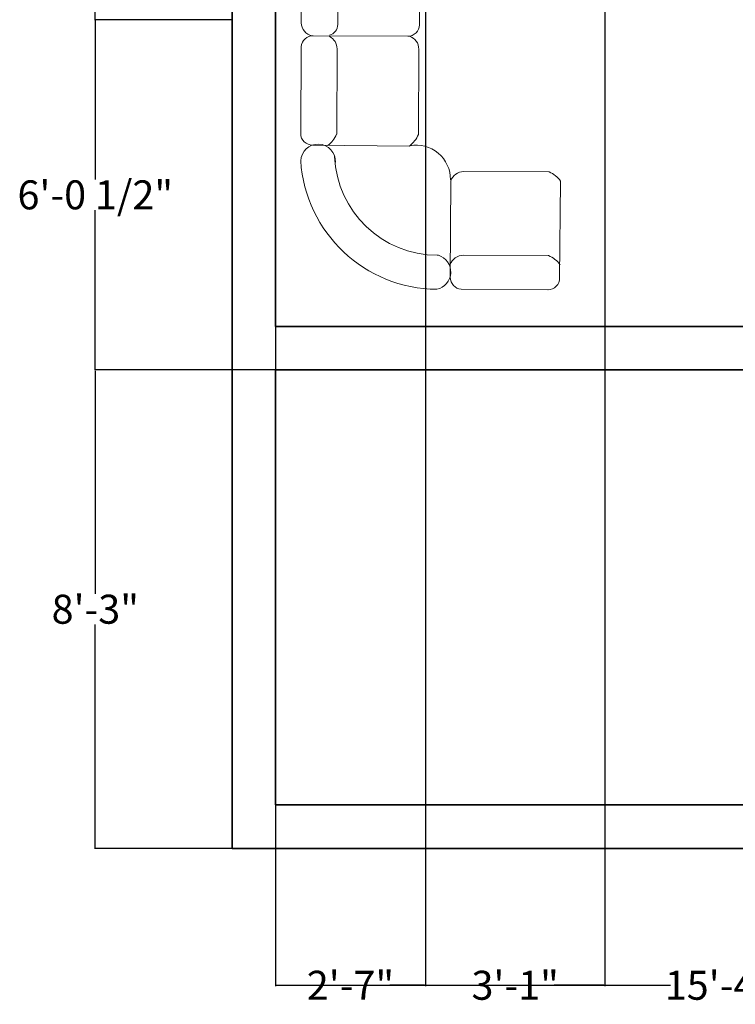
# Model space of a CAD drawing. Units: inches. Extents: x -26 to 575, y -18 to 513.
# Tile 1 of 28: x -26 to 122, y -13 to 191. Entities that reach past the tile are written whole.
import ezdxf

# ---------------------------------------------------------------- set-up
doc = ezdxf.new("R2010")
doc.units = ezdxf.units.IN
doc.header["$MEASUREMENT"] = 0
for name, color, linetype, lineweight in [('A-ANNO-DIMS', 2, 'Continuous', 18), ('A-WALL', 7, 'Continuous', 35), ('Furniture', 8, 'Continuous', 15)]:
    doc.layers.add(name, color=color, linetype=linetype, lineweight=lineweight)
doc.styles.get("Standard").update_dxf_attribs({"font": 'arial.ttf', "height": 6})
doc.dimstyles.get("Standard").update_dxf_attribs({"dimtxt": 6, "dimasz": 0.18, "dimexe": 0.18, "dimexo": 0.0625, "dimgap": 0.09, "dimtad": 0, "dimtih": 1, "dimtoh": 1, "dimzin": 0, "dimdsep": 46, "dimlunit": 3, "dimtxsty": 'Standard', "dimcen": 0.09, "dimadec": 0, "dimazin": 0, "dimtfac": 1, "dimtofl": 0, "dimtmove": 0, "dimatfit": 3, "dimfxl": 1, "dimtolj": 1, "dimtzin": 0, "dimarcsym": 0})

# ---------------------------------------------------------------- blocks, each defined once
blk = doc.blocks.new('SOFA-L-SECTIONAL')
for p, q in [((22.74, 97.99, -13.5), (2.82, 98.09, -13.5)), ((0.33, 95.83, -13.5), (0.23, 77.86, -13.5)), ((7.68, 77.72, -13.5), (7.77, 95.38, -13.5)), ((24.59, 77.63, -13.5), (24.69, 95.29, -13.5)), ((2.7, 75.47, -13.5), (22.72, 75.27, -13.5)), ((0.21, 72.7, -13.5), (0.12, 55.25, -13.5)), ((7.74, 68.12, -13.5), (7.76, 72.56, -13.5)), ((24.65, 68.03, -13.5), (24.67, 72.47, -13.5)), ((7.67, 54.9, -13.5), (7.74, 68.12, -13.5)), ((24.58, 54.81, -13.5), (24.65, 68.03, -13.5)), ((2.38, 52.55, -13.5), (22.19, 52.45, -13.5)), ((22.5, 52.45, -13.5), (2.58, 52.55, -13.5)), ((0.09, 50.29, -13.5), (0, 32.32, -13.5)), ((7.45, 32.18, -13.5), (7.54, 49.84, -13.5)), ((24.36, 32.09, -13.5), (24.45, 49.75, -13.5)), ((2.47, 29.93, -13.5), (22.49, 29.73, -13.5)), ((51.42, 24.36, -13.5), (33.76, 24.45, -13.5)), ((31.06, 22.5, -13.5), (30.96, 2.58, -13.5)), ((53.78, 22.49, -13.5), (53.58, 2.47, -13.5)), ((28.5, 7.13, -13.5), (28.26, 7.13, -13.5)), ((51.33, 7.05, -13.5), (33.67, 7.14, -13.5)), ((30.97, 5.19, -13.5), (30.97, 5.12, -13.5)), ((33.22, 0.09, -13.5), (51.19, 0, -13.5))]:
    blk.add_line(p, q)
for centre, radius, start, end in [((2.8, 95.6, -13.5), 2.49, 89.7045, 174.7543), ((4.96, 95.39, -13.5), 2.82, 359.7045, 63.7788), ((21.87, 95.31, -13.5), 2.82, 359.7045, 71.9933), ((2.61, 77.85, -13.5), 2.38, 179.7045, 272.1133), ((2.36, 80.01, -13.5), 5.79, 306.5883, 336.7547), ((19.27, 79.92, -13.5), 5.79, 306.5883, 336.7547), ((3.67, 72.1, -13.5), 3.51, 105.9725, 170.1982), ((4.8, 72.57, -13.5), 2.96, 359.7045, 69.9456), ((21.71, 72.48, -13.5), 2.96, 359.7045, 69.9456), ((2.84, 55.23, -13.5), 2.72, 179.7045, 260.1487), ((5.3, 54.91, -13.5), 2.37, 286.4623, 359.7335), ((22.21, 54.82, -13.5), 2.37, 269.7045, 359.7335), ((2.57, 50.06, -13.5), 2.49, 89.7045, 174.7543), ((4.72, 49.86, -13.5), 2.82, 359.7045, 63.7788), ((21.63, 49.77, -13.5), 2.82, 359.7045, 71.9933), ((2.38, 32.31, -13.5), 2.38, 179.7045, 272.1133), ((2.12, 34.47, -13.5), 5.79, 306.5883, 336.7547), ((19.04, 34.38, -13.5), 5.79, 306.5883, 336.7547), ((3.6, 26.52, -13.5), 3.6, 357.7166, 177.7166), ((23.89, 22.8, -13.5), 7.12, 359.7045, 100.3051), ((28.37, 28.51, -13.5), 28.42, 183.6915, 269.6528), ((28.37, 28.51, -13.5), 21.38, 182.6205, 269.7045), ((33.74, 21.63, -13.5), 2.82, 89.7045, 161.9933), ((49.13, 19.04, -13.5), 5.79, 36.5883, 66.7547), ((27.43, 3.65, -13.5), 3.64, 282.1306, 72.938), ((33.65, 4.32, -13.5), 2.82, 89.7045, 161.9933), ((49.04, 1.73, -13.5), 5.79, 36.5883, 66.7547), ((33.45, 2.57, -13.5), 2.49, 179.7045, 264.7543), ((51.2, 2.38, -13.5), 2.38, 269.7045, 2.1133)]:
    blk.add_arc(centre, radius, start, end)
blk = doc.blocks.new('*D28')
at = {"layer": 'A-ANNO-DIMS', "color": 0, "lineweight": -2, "transparency": 16777216}
for p, q in [((58.22, 466.45), (58.22, -8.97)), ((95.35, 466.45), (95.35, -8.97)), ((58.4, -8.79), (68.72, -8.79)), ((95.17, -8.79), (84.85, -8.79))]:
    blk.add_line(p, q, dxfattribs=at)
at = {"layer": 'A-ANNO-DIMS', "color": 0, "transparency": 16777216}
for points in [[(58.4, -8.76), (58.4, -8.82), (58.22, -8.79)], [(95.17, -8.76), (95.17, -8.82), (95.35, -8.79)]]:
    blk.add_solid(points, dxfattribs=at)
at = {"layer": 'Defpoints', "color": 0, "transparency": 16777216}
for p in [(58.22, 466.51), (95.35, 466.51), (95.35, -8.79)]:
    blk.add_point(p, dxfattribs=at)
at = {"layer": 'A-ANNO-DIMS', "color": 0, "transparency": 16777216, "insert": (76.79, -8.79), "char_height": 6, "attachment_point": 5}
blk.add_mtext('\\A1;3\'-1"', dxfattribs=at)
blk = doc.blocks.new('*D33')
at = {"layer": 'A-ANNO-DIMS', "color": 0, "lineweight": -2, "transparency": 16777216}
for p, q in [((27.11, 118.51), (-10.3, 118.51)), ((-10.12, 118.33), (-10.12, 72.16)), ((-10.12, 19.69), (-10.12, 65.85)), ((18.11, 19.51), (-10.3, 19.51))]:
    blk.add_line(p, q, dxfattribs=at)
at = {"layer": 'A-ANNO-DIMS', "color": 0, "transparency": 16777216}
for points in [[(-10.15, 118.33), (-10.09, 118.33), (-10.12, 118.51)], [(-10.15, 19.69), (-10.09, 19.69), (-10.12, 19.51)]]:
    blk.add_solid(points, dxfattribs=at)
at = {"layer": 'Defpoints', "color": 0, "transparency": 16777216}
for p in [(-10.12, 118.51), (27.18, 118.51), (18.18, 19.51)]:
    blk.add_point(p, dxfattribs=at)
at = {"layer": 'A-ANNO-DIMS', "color": 0, "transparency": 16777216, "insert": (-10.12, 69.01), "char_height": 6, "attachment_point": 5}
blk.add_mtext('\\A1;8\'-3"', dxfattribs=at)
blk = doc.blocks.new('*D36')
at = {"layer": 'A-ANNO-DIMS', "color": 0, "lineweight": -2, "transparency": 16777216}
for p, q in [((18.11, 267.49), (-10.3, 267.49)), ((-10.12, 267.31), (-10.12, 232.43)), ((-10.12, 191.16), (-10.12, 226.04)), ((18.11, 190.98), (-10.3, 190.98))]:
    blk.add_line(p, q, dxfattribs=at)
at = {"layer": 'A-ANNO-DIMS', "color": 0, "transparency": 16777216}
for points in [[(-10.15, 267.31), (-10.09, 267.31), (-10.12, 267.49)], [(-10.15, 191.16), (-10.09, 191.16), (-10.12, 190.98)]]:
    blk.add_solid(points, dxfattribs=at)
at = {"layer": 'Defpoints', "color": 0, "transparency": 16777216}
for p in [(-10.12, 267.49), (18.18, 267.49), (18.18, 190.98)]:
    blk.add_point(p, dxfattribs=at)
at = {"layer": 'A-ANNO-DIMS', "color": 0, "transparency": 16777216, "insert": (-10.12, 229.24), "char_height": 6, "attachment_point": 5}
blk.add_mtext('\\A1;6\'-4 1/2"', dxfattribs=at)
blk = doc.blocks.new('*D38')
at = {"layer": 'A-ANNO-DIMS', "color": 0, "lineweight": -2, "transparency": 16777216}
for p, q in [((18.11, 190.98), (-10.3, 190.98)), ((-10.12, 190.8), (-10.12, 157.94)), ((-10.12, 118.69), (-10.12, 151.55)), ((27.11, 118.51), (-10.3, 118.51))]:
    blk.add_line(p, q, dxfattribs=at)
at = {"layer": 'A-ANNO-DIMS', "color": 0, "transparency": 16777216}
for points in [[(-10.15, 190.8), (-10.09, 190.8), (-10.12, 190.98)], [(-10.15, 118.69), (-10.09, 118.69), (-10.12, 118.51)]]:
    blk.add_solid(points, dxfattribs=at)
at = {"layer": 'Defpoints', "color": 0, "transparency": 16777216}
for p in [(18.18, 190.98), (-10.12, 118.51), (27.18, 118.51)]:
    blk.add_point(p, dxfattribs=at)
at = {"layer": 'A-ANNO-DIMS', "color": 0, "transparency": 16777216, "insert": (-10.12, 154.74), "char_height": 6, "attachment_point": 5}
blk.add_mtext('\\A1;6\'-0 1/2"', dxfattribs=at)
blk = doc.blocks.new('*D40')
at = {"layer": 'A-ANNO-DIMS', "color": 0, "lineweight": -2, "transparency": 16777216}
for p, q in [((27.18, 118.45), (27.18, -8.97)), ((210.97, 118.45), (210.97, -8.97)), ((27.36, -8.79), (108.96, -8.79)), ((210.79, -8.79), (129.19, -8.79))]:
    blk.add_line(p, q, dxfattribs=at)
at = {"layer": 'A-ANNO-DIMS', "color": 0, "transparency": 16777216}
for points in [[(27.36, -8.76), (27.36, -8.82), (27.18, -8.79)], [(210.79, -8.76), (210.79, -8.82), (210.97, -8.79)]]:
    blk.add_solid(points, dxfattribs=at)
at = {"layer": 'Defpoints', "color": 0, "transparency": 16777216}
for p in [(27.18, 118.51), (210.97, 118.51), (27.18, -8.79)]:
    blk.add_point(p, dxfattribs=at)
at = {"layer": 'A-ANNO-DIMS', "color": 0, "transparency": 16777216, "insert": (119.07, -8.79), "char_height": 6, "attachment_point": 5}
blk.add_mtext('\\A1;15\'-4"', dxfattribs=at)
blk = doc.blocks.new('*D50')
at = {"layer": 'A-ANNO-DIMS', "color": 0, "lineweight": -2, "transparency": 16777216}
for p, q in [((27.18, 466.45), (27.18, -8.97)), ((58.22, 466.45), (58.22, -8.97)), ((27.36, -8.79), (34.58, -8.79)), ((58.04, -8.79), (50.82, -8.79))]:
    blk.add_line(p, q, dxfattribs=at)
at = {"layer": 'A-ANNO-DIMS', "color": 0, "transparency": 16777216}
for points in [[(27.36, -8.76), (27.36, -8.82), (27.18, -8.79)], [(58.04, -8.76), (58.04, -8.82), (58.22, -8.79)]]:
    blk.add_solid(points, dxfattribs=at)
at = {"layer": 'Defpoints', "color": 0, "transparency": 16777216}
for p in [(27.18, 466.51), (58.22, 466.51), (58.22, -8.79)]:
    blk.add_point(p, dxfattribs=at)
at = {"layer": 'A-ANNO-DIMS', "color": 0, "transparency": 16777216, "insert": (42.7, -8.79), "char_height": 6, "attachment_point": 5}
blk.add_mtext('\\A1;2\'-7"', dxfattribs=at)

msp = doc.modelspace()

# ---------------------------------------------------------------- linework, layer by layer
at = {"layer": 'A-WALL'}
for p, q in [((27.177, 330.008), (27.177, 127.508)), ((134.177, 127.508), (27.177, 127.508)), ((300.409, 118.508), (27.177, 118.508)), ((27.177, 118.508), (27.177, 28.508)), ((27.177, 28.508), (513.177, 28.508))]:
    msp.add_line(p, q, dxfattribs=at)
msp.add_lwpolyline([(18.177, 19.508), (522.177, 19.508), (522.177, 475.508), (18.177, 475.508)], close=True, dxfattribs=at)

# ---------------------------------------------------------------- block references
at = {"layer": 'Furniture'}
msp.add_blockref('SOFA-L-SECTIONAL', (32.395, 135.109), dxfattribs=at)

# ---------------------------------------------------------------- dimensions: what is measured, and where the dimension line sits
at = {"layer": 'A-ANNO-DIMS'}
for base, p1, p2, picture, middle in [((58.224, -8.792), (27.177, 466.508), (58.224, 466.508), '*D50', (42.7, -8.792)), ((95.349, -8.792), (58.224, 466.508), (95.349, 466.508), '*D28', (76.786, -8.792)), ((27.177, -8.792), (210.969, 118.508), (27.177, 118.508), '*D40', (119.073, -8.792))]:
    dim = msp.add_linear_dim(base=base, p1=p1, p2=p2, dimstyle='Standard', override={"dimdec": 1, "dimlfac": 1, "dimrnd": 0, "dimzin": 1, "dimdsep": 46, "dimlunit": 4, "dimfrac": 2}, dxfattribs=at)
    dim.commit()
    dim.dimension.update_dxf_attribs({"geometry": picture, "text_midpoint": middle})
for base, p1, p2, picture, middle in [((-10.123, 267.494), (18.177, 190.977), (18.177, 267.494), '*D36', (-10.123, 229.236)), ((-10.123, 118.508), (18.177, 190.977), (27.177, 118.508), '*D38', (-10.123, 154.743)), ((-10.123, 118.508), (18.177, 19.508), (27.177, 118.508), '*D33', (-10.123, 69.008))]:
    dim = msp.add_linear_dim(base=base, p1=p1, p2=p2, angle=90, dimstyle='Standard', override={"dimdec": 1, "dimlfac": 1, "dimrnd": 0, "dimzin": 1, "dimdsep": 46, "dimlunit": 4, "dimfrac": 2}, dxfattribs=at)
    dim.commit()
    dim.dimension.update_dxf_attribs({"geometry": picture, "text_midpoint": middle})

doc.saveas('drawing.dxf')
